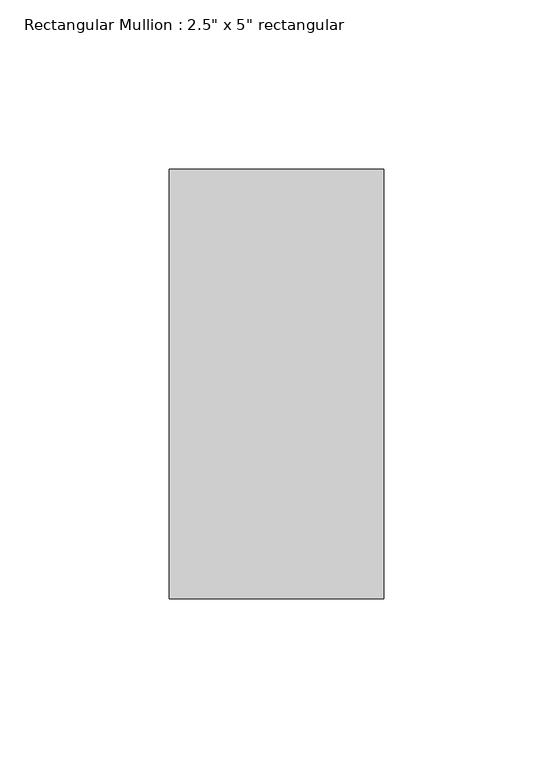
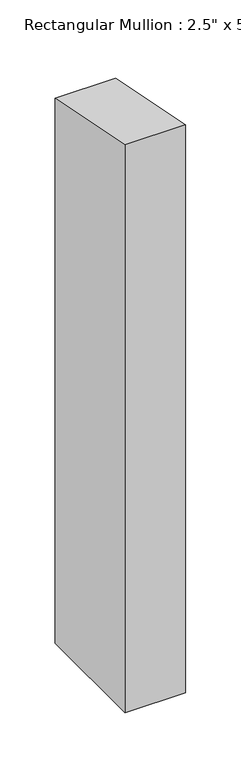
"""IFC4 building model written with IfcOpenShell, lengths in millimetres: member geometry."""

from ifc_helpers import new_model, si_unit, frame, origin, place, context, project, spatial, polyline, outline, extrude, source, transform, mapped, element, save


def member_9bbfae49(model_context):
    return source(origin(), model_context, "Body", "SweptSolid", [
        extrude(outline(polyline([(-63.5, 12.6309353), (63.5, -12.6309353), (63.5, -615.3845736), (-63.5, -615.3845736), (-63.5, 12.6309353)])), frame((-63.5, 0.0, 0.0), z_axis=(1.0, 0.0, 0.0), x_axis=(0.0, 1.0, 0.0)), (0.0, 0.0, 1.0), 63.5),
    ])


if __name__ == "__main__":
    model = new_model("IFC4")
    model_context = context("Model", 3, world=origin())
    ifc_project = project(units=[si_unit("LENGTHUNIT", "METRE", prefix="MILLI")], contexts=[model_context])
    site = spatial("IfcSite", under=ifc_project)
    building = spatial("IfcBuilding", under=site)
    placement = place(None, origin())
    member_shape = member_9bbfae49(model_context)
    element("IfcMember", 1, ObjectType="Rectangular Mullion : 2.5\" x 5\" rectangular", at=placement, inside=building, context=model_context, shape_type="MappedRepresentation", body=[
        mapped(member_shape, transform((0.0, 0.0, 0.0), x_axis=(1.0, 0.0, 0.0), y_axis=(0.0, 1.0, 0.0), z_axis=(0.0, 0.0, 1.0))),
    ])
    save(model, "model.ifc")

# Revit data of these elements
# Type "Rectangular Mullion : 2.5\" x 5\" rectangular"
#   built-in parameter 1007304 = 0.416667 (stored number, unit not read)
#   built-in parameter 1007301 = 0.104167 (stored number, unit not read)
#   built-in parameter 1007300 = 0.104167 (stored number, unit not read)
# Element 1 (IfcMember, "Rectangular Mullion : 2.5\" x 5\" rectangular")
#   Materials on its faces: "Iron, Ductile"
# Materials
#   "Iron, Ductile": class "Metal", colour RGB 0 0 0, transparency 0, Description = "Ductile cast iron", Cost = 0
